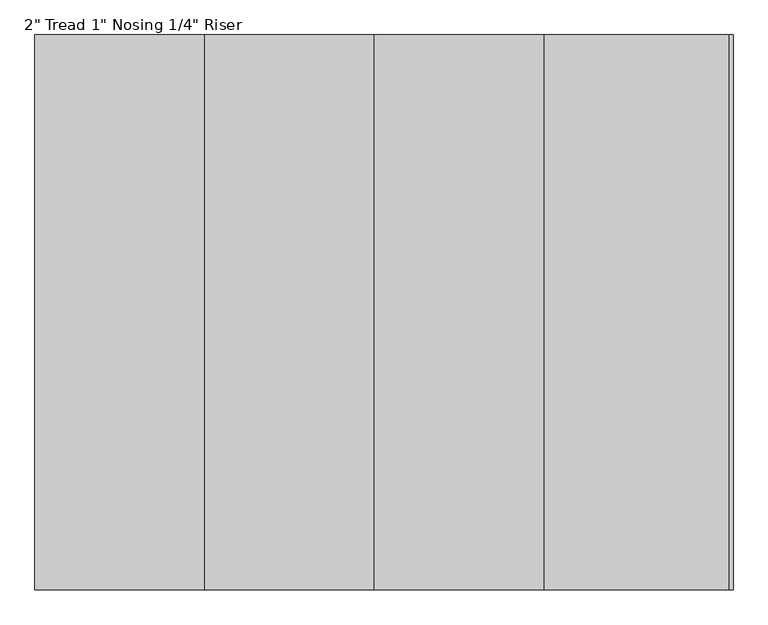
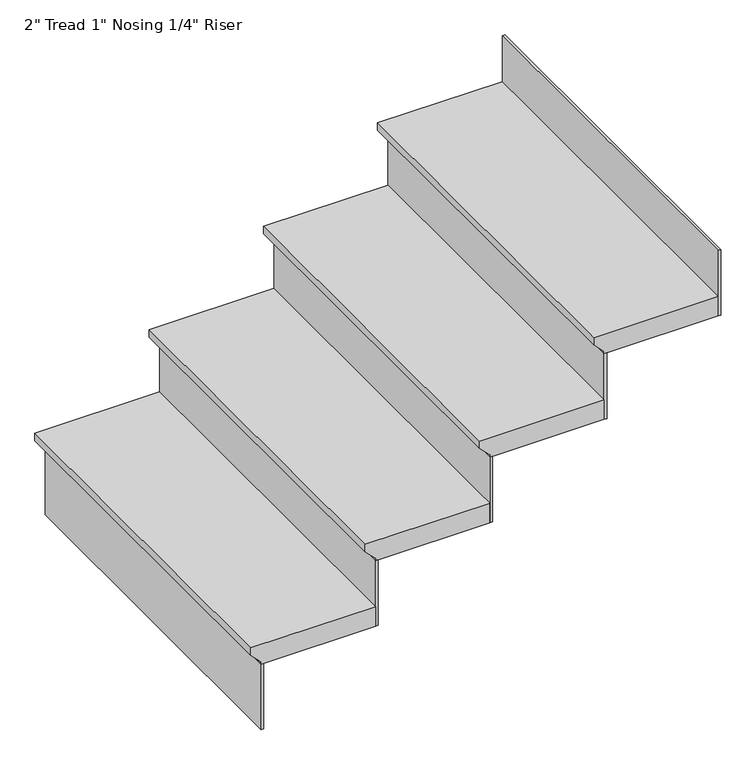
"""IFC4 building model written with IfcOpenShell, lengths in millimetres: stair flight geometry."""

from ifc_helpers import new_model, si_unit, frame, origin, place, context, project, spatial, polyline, outline, extrude, source, transform, mapped, element, save


def stair_flight_5ad97bb6(model_context):
    return source(origin(), model_context, "Body", "SweptSolid", [
        extrude(outline(polyline([(2370.6666667, -16645.533929), (2370.6666667, -16950.333929), (2351.6166667, -16950.333929), (2326.2166667, -16924.933929), (2319.8666667, -16924.933929), (2319.8666667, -16645.533929), (2370.6666667, -16645.533929)])), frame((0.0, 16271.1159704, 0.0), z_axis=(0.0, 1.0, 0.0), x_axis=(0.0, 0.0, 1.0)), (0.0, 0.0, 1.0), 914.4),
        extrude(outline(polyline([(-16918.583929, 16271.1159704), (-16924.933929, 16271.1159704), (-16924.933929, 17185.5159704), (-16918.583929, 17185.5159704), (-16918.583929, 16271.1159704)])), frame((0.0, 0.0, 2150.5333333), z_axis=(0.0, 0.0, 1.0), x_axis=(1.0, 0.0, 0.0)), (0.0, 0.0, 1.0), 169.3333333),
        extrude(outline(polyline([(-16639.183929, 16271.1159704), (-16645.533929, 16271.1159704), (-16645.533929, 17185.5159704), (-16639.183929, 17185.5159704), (-16639.183929, 16271.1159704)])), frame((0.0, 0.0, 2319.8666667), z_axis=(0.0, 0.0, 1.0), x_axis=(1.0, 0.0, 0.0)), (0.0, 0.0, 1.0), 169.3333333),
        extrude(outline(polyline([(2540.0, -16366.133929), (2540.0, -16670.933929), (2520.95, -16670.933929), (2495.55, -16645.533929), (2489.2, -16645.533929), (2489.2, -16366.133929), (2540.0, -16366.133929)])), frame((0.0, 16271.1159704, 0.0), z_axis=(0.0, 1.0, 0.0), x_axis=(0.0, 0.0, 1.0)), (0.0, 0.0, 1.0), 914.4),
        extrude(outline(polyline([(-16359.783929, 16271.1159704), (-16366.133929, 16271.1159704), (-16366.133929, 17185.5159704), (-16359.783929, 17185.5159704), (-16359.783929, 16271.1159704)])), frame((0.0, 0.0, 2489.2), z_axis=(0.0, 0.0, 1.0), x_axis=(1.0, 0.0, 0.0)), (0.0, 0.0, 1.0), 169.3333333),
        extrude(outline(polyline([(2709.3333333, -16086.733929), (2709.3333333, -16391.533929), (2690.2833333, -16391.533929), (2664.8833333, -16366.133929), (2658.5333333, -16366.133929), (2658.5333333, -16086.733929), (2709.3333333, -16086.733929)])), frame((0.0, 16271.1159704, 0.0), z_axis=(0.0, 1.0, 0.0), x_axis=(0.0, 0.0, 1.0)), (0.0, 0.0, 1.0), 914.4),
        extrude(outline(polyline([(-16080.383929, 16271.1159704), (-16086.733929, 16271.1159704), (-16086.733929, 17185.5159704), (-16080.383929, 17185.5159704), (-16080.383929, 16271.1159704)])), frame((0.0, 0.0, 2658.5333333), z_axis=(0.0, 0.0, 1.0), x_axis=(1.0, 0.0, 0.0)), (0.0, 0.0, 1.0), 169.3333333),
        extrude(outline(polyline([(-15800.983929, 16271.1159704), (-15807.333929, 16271.1159704), (-15807.333929, 17185.5159704), (-15800.983929, 17185.5159704), (-15800.983929, 16271.1159704)])), frame((0.0, 0.0, 2827.8666667), z_axis=(0.0, 0.0, 1.0), x_axis=(1.0, 0.0, 0.0)), (0.0, 0.0, 1.0), 169.3333333),
        extrude(outline(polyline([(2878.6666667, -15807.333929), (2878.6666667, -16112.133929), (2859.6166667, -16112.133929), (2834.2166667, -16086.733929), (2827.8666667, -16086.733929), (2827.8666667, -15807.333929), (2878.6666667, -15807.333929)])), frame((0.0, 16271.1159704, 0.0), z_axis=(0.0, 1.0, 0.0), x_axis=(0.0, 0.0, 1.0)), (0.0, 0.0, 1.0), 914.4),
    ])


if __name__ == "__main__":
    model = new_model("IFC4")
    model_context = context("Model", 3, world=origin())
    ifc_project = project(units=[si_unit("LENGTHUNIT", "METRE", prefix="MILLI")], contexts=[model_context])
    site = spatial("IfcSite", under=ifc_project)
    building = spatial("IfcBuilding", under=site)
    placement = place(None, origin())
    stair_flight_shape = stair_flight_5ad97bb6(model_context)
    element("IfcStairFlight", 1, ObjectType="2\" Tread 1\" Nosing 1/4\" Riser", at=placement, inside=building, context=model_context, shape_type="MappedRepresentation", body=[
        mapped(stair_flight_shape, transform((0.0, 0.0, 0.0), x_axis=(1.0, 0.0, 0.0), y_axis=(0.0, 1.0, 0.0), z_axis=(0.0, 0.0, 1.0))),
    ])
    save(model, "model.ifc")
